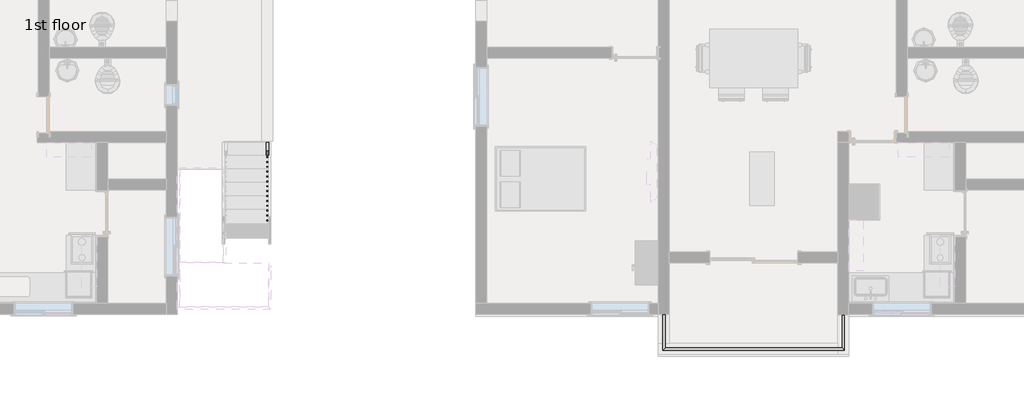
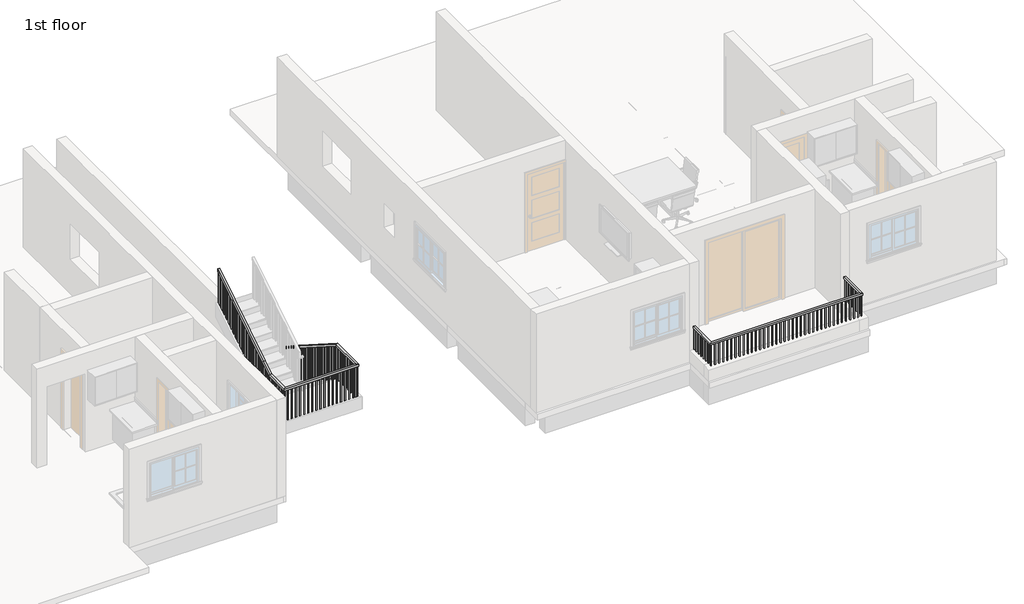
# One storey, part 5 of 8: 2 railings.
"""IFC4 building model written with IfcOpenShell, lengths in millimetres."""

from ifc_helpers import new_model, si_unit, frame, origin, place, context, project, spatial, polyline, outline, extrude, faceted_brep, element, save

model = new_model("IFC4")

# Units and contexts
model_context = context("Model", 3, world=origin())
ifc_project = project(units=[si_unit("LENGTHUNIT", "METRE", prefix="MILLI")], contexts=[model_context])

# Site, building, storey
site = spatial("IfcSite", under=ifc_project)
building = spatial("IfcBuilding", under=site)
storey = spatial("IfcBuildingStorey", under=building, Name="1st floor", Elevation=3810.0)

# Railings
placement = place(None, origin())
element("IfcRailing", 1, ObjectType="Handrail - Rectangular", at=placement, inside=storey, context=model_context, shape_type="SolidModel", body=[
    faceted_brep([(-2736.9993763, -1023.9064015, 4902.2), (-2736.9993763, -1023.9064015, 4841.986276), (-2787.7993763, -1023.9064015, 4841.986276), (-2787.7993763, -1023.9064015, 4902.2), (-2736.9993763, -3538.5064015, 6502.4), (-2736.9993763, -3553.2993964, 6451.6), (-2787.7993763, -3553.2993964, 6451.6), (-2787.7993763, -3538.5064015, 6502.4), (-2736.9993763, -4452.9064015, 6502.4), (-2736.9993763, -4452.9064015, 6451.6), (-2787.7993763, -4402.1064015, 6451.6), (-2787.7993763, -4402.1064015, 6502.4), (-4591.1993763, -4452.9064015, 6502.4), (-4591.1993763, -4452.9064015, 6451.6), (-4540.3993763, -4402.1064015, 6451.6), (-4540.3993763, -4402.1064015, 6502.4), (-4591.1993763, -3817.9064015, 6502.4), (-4591.1993763, -3803.1134066, 6451.6), (-4540.3993763, -3803.1134066, 6451.6), (-4540.3993763, -3817.9064015, 6502.4), (-4591.1993763, -3538.5064015, 6680.2), (-4591.1993763, -3511.2331265, 6637.3419964), (-4540.3993763, -3511.2331265, 6637.3419964), (-4540.3993763, -3538.5064015, 6680.2), (-4591.1993763, -1582.7064015, 7924.8), (-4540.3993763, -1582.7064015, 7924.8), (-4540.3993763, -1582.7064015, 7864.586276), (-4591.1993763, -1582.7064015, 7864.586276)], [[[0, 1, 2, 3]], [[1, 0, 4, 5]], [[2, 1, 5, 6]], [[3, 2, 6, 7]], [[0, 3, 7, 4]], [[5, 4, 8, 9]], [[6, 5, 9, 10]], [[7, 6, 10, 11]], [[4, 7, 11, 8]], [[9, 8, 12, 13]], [[10, 9, 13, 14]], [[11, 10, 14, 15]], [[8, 11, 15, 12]], [[13, 12, 16, 17]], [[14, 13, 17, 18]], [[15, 14, 18, 19]], [[12, 15, 19, 16]], [[17, 16, 20, 21]], [[18, 17, 21, 22]], [[19, 18, 22, 23]], [[16, 19, 23, 20]], [[24, 25, 26, 27]], [[21, 20, 24, 27]], [[22, 21, 27, 26]], [[23, 22, 26, 25]], [[20, 23, 25, 24]]]),
    extrude(outline(polyline([(-1598.5814015, 7854.4840032), (-1598.5814015, 6832.6), (-1617.6314015, 6832.6), (-1617.6314015, 7842.361276), (-1598.5814015, 7854.4840032)])), frame((-4575.3243763, 0.0, 0.0), z_axis=(1.0, 0.0, 0.0), x_axis=(0.0, 1.0, 0.0)), (0.0, 0.0, 1.0), 19.05),
    extrude(outline(polyline([(-1700.1814015, 7789.8294578), (-1700.1814015, 6832.6), (-1719.2314015, 6832.6), (-1719.2314015, 7777.7067305), (-1700.1814015, 7789.8294578)])), frame((-4575.3243763, 0.0, 0.0), z_axis=(1.0, 0.0, 0.0), x_axis=(0.0, 1.0, 0.0)), (0.0, 0.0, 1.0), 19.05),
    extrude(outline(polyline([(-1801.7814015, 7725.1749123), (-1801.7814015, 6832.6), (-1820.8314015, 6832.6), (-1820.8314015, 7713.0521851), (-1801.7814015, 7725.1749123)])), frame((-4575.3243763, 0.0, 0.0), z_axis=(1.0, 0.0, 0.0), x_axis=(0.0, 1.0, 0.0)), (0.0, 0.0, 1.0), 19.05),
    extrude(outline(polyline([(-1903.3814015, 7660.5203669), (-1903.3814015, 6654.8), (-1922.4314015, 6654.8), (-1922.4314015, 7648.3976396), (-1903.3814015, 7660.5203669)])), frame((-4575.3243763, 0.0, 0.0), z_axis=(1.0, 0.0, 0.0), x_axis=(0.0, 1.0, 0.0)), (0.0, 0.0, 1.0), 19.05),
    extrude(outline(polyline([(-2004.9814015, 7595.8658214), (-2004.9814015, 6654.8), (-2024.0314015, 6654.8), (-2024.0314015, 7583.7430941), (-2004.9814015, 7595.8658214)])), frame((-4575.3243763, 0.0, 0.0), z_axis=(1.0, 0.0, 0.0), x_axis=(0.0, 1.0, 0.0)), (0.0, 0.0, 1.0), 19.05),
    extrude(outline(polyline([(-2106.5814015, 7531.211276), (-2106.5814015, 6654.8), (-2125.6314015, 6654.8), (-2125.6314015, 7519.0885487), (-2106.5814015, 7531.211276)])), frame((-4575.3243763, 0.0, 0.0), z_axis=(1.0, 0.0, 0.0), x_axis=(0.0, 1.0, 0.0)), (0.0, 0.0, 1.0), 19.05),
    extrude(outline(polyline([(-2208.1814015, 7466.5567305), (-2208.1814015, 6477.0), (-2227.2314015, 6477.0), (-2227.2314015, 7454.4340032), (-2208.1814015, 7466.5567305)])), frame((-4575.3243763, 0.0, 0.0), z_axis=(1.0, 0.0, 0.0), x_axis=(0.0, 1.0, 0.0)), (0.0, 0.0, 1.0), 19.05),
    extrude(outline(polyline([(-2309.7814015, 7401.9021851), (-2309.7814015, 6477.0), (-2328.8314015, 6477.0), (-2328.8314015, 7389.7794578), (-2309.7814015, 7401.9021851)])), frame((-4575.3243763, 0.0, 0.0), z_axis=(1.0, 0.0, 0.0), x_axis=(0.0, 1.0, 0.0)), (0.0, 0.0, 1.0), 19.05),
    extrude(outline(polyline([(-2411.3814015, 7337.2476396), (-2411.3814015, 6477.0), (-2430.4314015, 6477.0), (-2430.4314015, 7325.1249123), (-2411.3814015, 7337.2476396)])), frame((-4575.3243763, 0.0, 0.0), z_axis=(1.0, 0.0, 0.0), x_axis=(0.0, 1.0, 0.0)), (0.0, 0.0, 1.0), 19.05),
    extrude(outline(polyline([(-2512.9814015, 7272.5930941), (-2512.9814015, 6299.2), (-2532.0314015, 6299.2), (-2532.0314015, 7260.4703669), (-2512.9814015, 7272.5930941)])), frame((-4575.3243763, 0.0, 0.0), z_axis=(1.0, 0.0, 0.0), x_axis=(0.0, 1.0, 0.0)), (0.0, 0.0, 1.0), 19.05),
    extrude(outline(polyline([(-2614.5814015, 7207.9385487), (-2614.5814015, 6299.2), (-2633.6314015, 6299.2), (-2633.6314015, 7195.8158214), (-2614.5814015, 7207.9385487)])), frame((-4575.3243763, 0.0, 0.0), z_axis=(1.0, 0.0, 0.0), x_axis=(0.0, 1.0, 0.0)), (0.0, 0.0, 1.0), 19.05),
    extrude(outline(polyline([(-2716.1814015, 7143.2840032), (-2716.1814015, 6121.4), (-2735.2314015, 6121.4), (-2735.2314015, 7131.161276), (-2716.1814015, 7143.2840032)])), frame((-4575.3243763, 0.0, 0.0), z_axis=(1.0, 0.0, 0.0), x_axis=(0.0, 1.0, 0.0)), (0.0, 0.0, 1.0), 19.05),
    extrude(outline(polyline([(-2817.7814015, 7078.6294578), (-2817.7814015, 6121.4), (-2836.8314015, 6121.4), (-2836.8314015, 7066.5067305), (-2817.7814015, 7078.6294578)])), frame((-4575.3243763, 0.0, 0.0), z_axis=(1.0, 0.0, 0.0), x_axis=(0.0, 1.0, 0.0)), (0.0, 0.0, 1.0), 19.05),
    extrude(outline(polyline([(-2919.3814015, 7013.9749123), (-2919.3814015, 6121.4), (-2938.4314015, 6121.4), (-2938.4314015, 7001.8521851), (-2919.3814015, 7013.9749123)])), frame((-4575.3243763, 0.0, 0.0), z_axis=(1.0, 0.0, 0.0), x_axis=(0.0, 1.0, 0.0)), (0.0, 0.0, 1.0), 19.05),
    extrude(outline(polyline([(-3020.9814015, 6949.3203669), (-3020.9814015, 5943.6), (-3040.0314015, 5943.6), (-3040.0314015, 6937.1976396), (-3020.9814015, 6949.3203669)])), frame((-4575.3243763, 0.0, 0.0), z_axis=(1.0, 0.0, 0.0), x_axis=(0.0, 1.0, 0.0)), (0.0, 0.0, 1.0), 19.05),
    extrude(outline(polyline([(-3122.5814015, 6884.6658214), (-3122.5814015, 5943.6), (-3141.6314015, 5943.6), (-3141.6314015, 6872.5430941), (-3122.5814015, 6884.6658214)])), frame((-4575.3243763, 0.0, 0.0), z_axis=(1.0, 0.0, 0.0), x_axis=(0.0, 1.0, 0.0)), (0.0, 0.0, 1.0), 19.05),
    extrude(outline(polyline([(-3224.1814015, 6820.011276), (-3224.1814015, 5943.6), (-3243.2314015, 5943.6), (-3243.2314015, 6807.8885487), (-3224.1814015, 6820.011276)])), frame((-4575.3243763, 0.0, 0.0), z_axis=(1.0, 0.0, 0.0), x_axis=(0.0, 1.0, 0.0)), (0.0, 0.0, 1.0), 19.05),
    extrude(outline(polyline([(-3325.7814015, 6755.3567305), (-3325.7814015, 5765.8), (-3344.8314015, 5765.8), (-3344.8314015, 6743.2340032), (-3325.7814015, 6755.3567305)])), frame((-4575.3243763, 0.0, 0.0), z_axis=(1.0, 0.0, 0.0), x_axis=(0.0, 1.0, 0.0)), (0.0, 0.0, 1.0), 19.05),
    extrude(outline(polyline([(-3427.3814015, 6690.7021851), (-3427.3814015, 5765.8), (-3446.4314015, 5765.8), (-3446.4314015, 6678.5794578), (-3427.3814015, 6690.7021851)])), frame((-4575.3243763, 0.0, 0.0), z_axis=(1.0, 0.0, 0.0), x_axis=(0.0, 1.0, 0.0)), (0.0, 0.0, 1.0), 19.05),
    extrude(outline(polyline([(-3605.1814015, 6577.5567305), (-3605.1814015, 5588.0), (-3624.2314015, 5588.0), (-3624.2314015, 6565.4340032), (-3605.1814015, 6577.5567305)])), frame((-4575.3243763, 0.0, 0.0), z_axis=(1.0, 0.0, 0.0), x_axis=(0.0, 1.0, 0.0)), (0.0, 0.0, 1.0), 19.05),
    extrude(outline(polyline([(-3706.7814015, 6512.9021851), (-3706.7814015, 5588.0), (-3725.8314015, 5588.0), (-3725.8314015, 6500.7794578), (-3706.7814015, 6512.9021851)])), frame((-4575.3243763, 0.0, 0.0), z_axis=(1.0, 0.0, 0.0), x_axis=(0.0, 1.0, 0.0)), (0.0, 0.0, 1.0), 19.05),
    extrude(outline(polyline([(-4575.3243763, -3827.4314015), (-4575.3243763, -3808.3814015), (-4556.2743763, -3808.3814015), (-4556.2743763, -3827.4314015), (-4575.3243763, -3827.4314015)])), frame((0.0, 0.0, 5588.0), z_axis=(0.0, 0.0, 1.0), x_axis=(1.0, 0.0, 0.0)), (0.0, 0.0, 1.0), 863.6),
    extrude(outline(polyline([(-4575.3243763, -3929.0314015), (-4575.3243763, -3909.9814015), (-4556.2743763, -3909.9814015), (-4556.2743763, -3929.0314015), (-4575.3243763, -3929.0314015)])), frame((0.0, 0.0, 5588.0), z_axis=(0.0, 0.0, 1.0), x_axis=(1.0, 0.0, 0.0)), (0.0, 0.0, 1.0), 863.6),
    extrude(outline(polyline([(-4575.3243763, -4030.6314015), (-4575.3243763, -4011.5814015), (-4556.2743763, -4011.5814015), (-4556.2743763, -4030.6314015), (-4575.3243763, -4030.6314015)])), frame((0.0, 0.0, 5588.0), z_axis=(0.0, 0.0, 1.0), x_axis=(1.0, 0.0, 0.0)), (0.0, 0.0, 1.0), 863.6),
    extrude(outline(polyline([(-4575.3243763, -4132.2314015), (-4575.3243763, -4113.1814015), (-4556.2743763, -4113.1814015), (-4556.2743763, -4132.2314015), (-4575.3243763, -4132.2314015)])), frame((0.0, 0.0, 5588.0), z_axis=(0.0, 0.0, 1.0), x_axis=(1.0, 0.0, 0.0)), (0.0, 0.0, 1.0), 863.6),
    extrude(outline(polyline([(-4575.3243763, -4233.8314015), (-4575.3243763, -4214.7814015), (-4556.2743763, -4214.7814015), (-4556.2743763, -4233.8314015), (-4575.3243763, -4233.8314015)])), frame((0.0, 0.0, 5588.0), z_axis=(0.0, 0.0, 1.0), x_axis=(1.0, 0.0, 0.0)), (0.0, 0.0, 1.0), 863.6),
    extrude(outline(polyline([(-4575.3243763, -4335.4314015), (-4575.3243763, -4316.3814015), (-4556.2743763, -4316.3814015), (-4556.2743763, -4335.4314015), (-4575.3243763, -4335.4314015)])), frame((0.0, 0.0, 5588.0), z_axis=(0.0, 0.0, 1.0), x_axis=(1.0, 0.0, 0.0)), (0.0, 0.0, 1.0), 863.6),
    extrude(outline(polyline([(-4480.0743763, -4437.0314015), (-4499.1243763, -4437.0314015), (-4499.1243763, -4417.9814015), (-4480.0743763, -4417.9814015), (-4480.0743763, -4437.0314015)])), frame((0.0, 0.0, 5588.0), z_axis=(0.0, 0.0, 1.0), x_axis=(1.0, 0.0, 0.0)), (0.0, 0.0, 1.0), 863.6),
    extrude(outline(polyline([(-4378.4743763, -4437.0314015), (-4397.5243763, -4437.0314015), (-4397.5243763, -4417.9814015), (-4378.4743763, -4417.9814015), (-4378.4743763, -4437.0314015)])), frame((0.0, 0.0, 5588.0), z_axis=(0.0, 0.0, 1.0), x_axis=(1.0, 0.0, 0.0)), (0.0, 0.0, 1.0), 863.6),
    extrude(outline(polyline([(-4276.8743763, -4437.0314015), (-4295.9243763, -4437.0314015), (-4295.9243763, -4417.9814015), (-4276.8743763, -4417.9814015), (-4276.8743763, -4437.0314015)])), frame((0.0, 0.0, 5588.0), z_axis=(0.0, 0.0, 1.0), x_axis=(1.0, 0.0, 0.0)), (0.0, 0.0, 1.0), 863.6),
    extrude(outline(polyline([(-4175.2743763, -4437.0314015), (-4194.3243763, -4437.0314015), (-4194.3243763, -4417.9814015), (-4175.2743763, -4417.9814015), (-4175.2743763, -4437.0314015)])), frame((0.0, 0.0, 5588.0), z_axis=(0.0, 0.0, 1.0), x_axis=(1.0, 0.0, 0.0)), (0.0, 0.0, 1.0), 863.6),
    extrude(outline(polyline([(-4073.6743763, -4437.0314015), (-4092.7243763, -4437.0314015), (-4092.7243763, -4417.9814015), (-4073.6743763, -4417.9814015), (-4073.6743763, -4437.0314015)])), frame((0.0, 0.0, 5588.0), z_axis=(0.0, 0.0, 1.0), x_axis=(1.0, 0.0, 0.0)), (0.0, 0.0, 1.0), 863.6),
    extrude(outline(polyline([(-3972.0743763, -4437.0314015), (-3991.1243763, -4437.0314015), (-3991.1243763, -4417.9814015), (-3972.0743763, -4417.9814015), (-3972.0743763, -4437.0314015)])), frame((0.0, 0.0, 5588.0), z_axis=(0.0, 0.0, 1.0), x_axis=(1.0, 0.0, 0.0)), (0.0, 0.0, 1.0), 863.6),
    extrude(outline(polyline([(-3870.4743763, -4437.0314015), (-3889.5243763, -4437.0314015), (-3889.5243763, -4417.9814015), (-3870.4743763, -4417.9814015), (-3870.4743763, -4437.0314015)])), frame((0.0, 0.0, 5588.0), z_axis=(0.0, 0.0, 1.0), x_axis=(1.0, 0.0, 0.0)), (0.0, 0.0, 1.0), 863.6),
    extrude(outline(polyline([(-3768.8743763, -4437.0314015), (-3787.9243763, -4437.0314015), (-3787.9243763, -4417.9814015), (-3768.8743763, -4417.9814015), (-3768.8743763, -4437.0314015)])), frame((0.0, 0.0, 5588.0), z_axis=(0.0, 0.0, 1.0), x_axis=(1.0, 0.0, 0.0)), (0.0, 0.0, 1.0), 863.6),
    extrude(outline(polyline([(-3667.2743763, -4437.0314015), (-3686.3243763, -4437.0314015), (-3686.3243763, -4417.9814015), (-3667.2743763, -4417.9814015), (-3667.2743763, -4437.0314015)])), frame((0.0, 0.0, 5588.0), z_axis=(0.0, 0.0, 1.0), x_axis=(1.0, 0.0, 0.0)), (0.0, 0.0, 1.0), 863.6),
    extrude(outline(polyline([(-3565.6743763, -4437.0314015), (-3584.7243763, -4437.0314015), (-3584.7243763, -4417.9814015), (-3565.6743763, -4417.9814015), (-3565.6743763, -4437.0314015)])), frame((0.0, 0.0, 5588.0), z_axis=(0.0, 0.0, 1.0), x_axis=(1.0, 0.0, 0.0)), (0.0, 0.0, 1.0), 863.6),
    extrude(outline(polyline([(-3464.0743763, -4437.0314015), (-3483.1243763, -4437.0314015), (-3483.1243763, -4417.9814015), (-3464.0743763, -4417.9814015), (-3464.0743763, -4437.0314015)])), frame((0.0, 0.0, 5588.0), z_axis=(0.0, 0.0, 1.0), x_axis=(1.0, 0.0, 0.0)), (0.0, 0.0, 1.0), 863.6),
    extrude(outline(polyline([(-3362.4743763, -4437.0314015), (-3381.5243763, -4437.0314015), (-3381.5243763, -4417.9814015), (-3362.4743763, -4417.9814015), (-3362.4743763, -4437.0314015)])), frame((0.0, 0.0, 5588.0), z_axis=(0.0, 0.0, 1.0), x_axis=(1.0, 0.0, 0.0)), (0.0, 0.0, 1.0), 863.6),
    extrude(outline(polyline([(-3260.8743763, -4437.0314015), (-3279.9243763, -4437.0314015), (-3279.9243763, -4417.9814015), (-3260.8743763, -4417.9814015), (-3260.8743763, -4437.0314015)])), frame((0.0, 0.0, 5588.0), z_axis=(0.0, 0.0, 1.0), x_axis=(1.0, 0.0, 0.0)), (0.0, 0.0, 1.0), 863.6),
    extrude(outline(polyline([(-3159.2743763, -4437.0314015), (-3178.3243763, -4437.0314015), (-3178.3243763, -4417.9814015), (-3159.2743763, -4417.9814015), (-3159.2743763, -4437.0314015)])), frame((0.0, 0.0, 5588.0), z_axis=(0.0, 0.0, 1.0), x_axis=(1.0, 0.0, 0.0)), (0.0, 0.0, 1.0), 863.6),
    extrude(outline(polyline([(-3057.6743763, -4437.0314015), (-3076.7243763, -4437.0314015), (-3076.7243763, -4417.9814015), (-3057.6743763, -4417.9814015), (-3057.6743763, -4437.0314015)])), frame((0.0, 0.0, 5588.0), z_axis=(0.0, 0.0, 1.0), x_axis=(1.0, 0.0, 0.0)), (0.0, 0.0, 1.0), 863.6),
    extrude(outline(polyline([(-2956.0743763, -4437.0314015), (-2975.1243763, -4437.0314015), (-2975.1243763, -4417.9814015), (-2956.0743763, -4417.9814015), (-2956.0743763, -4437.0314015)])), frame((0.0, 0.0, 5588.0), z_axis=(0.0, 0.0, 1.0), x_axis=(1.0, 0.0, 0.0)), (0.0, 0.0, 1.0), 863.6),
    extrude(outline(polyline([(-2854.4743763, -4437.0314015), (-2873.5243763, -4437.0314015), (-2873.5243763, -4417.9814015), (-2854.4743763, -4417.9814015), (-2854.4743763, -4437.0314015)])), frame((0.0, 0.0, 5588.0), z_axis=(0.0, 0.0, 1.0), x_axis=(1.0, 0.0, 0.0)), (0.0, 0.0, 1.0), 863.6),
    extrude(outline(polyline([(-2752.8743763, -4341.7814015), (-2752.8743763, -4360.8314015), (-2771.9243763, -4360.8314015), (-2771.9243763, -4341.7814015), (-2752.8743763, -4341.7814015)])), frame((0.0, 0.0, 5588.0), z_axis=(0.0, 0.0, 1.0), x_axis=(1.0, 0.0, 0.0)), (0.0, 0.0, 1.0), 863.6),
    extrude(outline(polyline([(-2752.8743763, -4240.1814015), (-2752.8743763, -4259.2314015), (-2771.9243763, -4259.2314015), (-2771.9243763, -4240.1814015), (-2752.8743763, -4240.1814015)])), frame((0.0, 0.0, 5588.0), z_axis=(0.0, 0.0, 1.0), x_axis=(1.0, 0.0, 0.0)), (0.0, 0.0, 1.0), 863.6),
    extrude(outline(polyline([(-2752.8743763, -4138.5814015), (-2752.8743763, -4157.6314015), (-2771.9243763, -4157.6314015), (-2771.9243763, -4138.5814015), (-2752.8743763, -4138.5814015)])), frame((0.0, 0.0, 5588.0), z_axis=(0.0, 0.0, 1.0), x_axis=(1.0, 0.0, 0.0)), (0.0, 0.0, 1.0), 863.6),
    extrude(outline(polyline([(-2752.8743763, -4036.9814015), (-2752.8743763, -4056.0314015), (-2771.9243763, -4056.0314015), (-2771.9243763, -4036.9814015), (-2752.8743763, -4036.9814015)])), frame((0.0, 0.0, 5588.0), z_axis=(0.0, 0.0, 1.0), x_axis=(1.0, 0.0, 0.0)), (0.0, 0.0, 1.0), 863.6),
    extrude(outline(polyline([(-2752.8743763, -3935.3814015), (-2752.8743763, -3954.4314015), (-2771.9243763, -3954.4314015), (-2771.9243763, -3935.3814015), (-2752.8743763, -3935.3814015)])), frame((0.0, 0.0, 5588.0), z_axis=(0.0, 0.0, 1.0), x_axis=(1.0, 0.0, 0.0)), (0.0, 0.0, 1.0), 863.6),
    extrude(outline(polyline([(-2752.8743763, -3833.7814015), (-2752.8743763, -3852.8314015), (-2771.9243763, -3852.8314015), (-2771.9243763, -3833.7814015), (-2752.8743763, -3833.7814015)])), frame((0.0, 0.0, 5588.0), z_axis=(0.0, 0.0, 1.0), x_axis=(1.0, 0.0, 0.0)), (0.0, 0.0, 1.0), 863.6),
    extrude(outline(polyline([(-2752.8743763, -3732.1814015), (-2752.8743763, -3751.2314015), (-2771.9243763, -3751.2314015), (-2771.9243763, -3732.1814015), (-2752.8743763, -3732.1814015)])), frame((0.0, 0.0, 5588.0), z_axis=(0.0, 0.0, 1.0), x_axis=(1.0, 0.0, 0.0)), (0.0, 0.0, 1.0), 863.6),
    extrude(outline(polyline([(-2752.8743763, -3630.5814015), (-2752.8743763, -3649.6314015), (-2771.9243763, -3649.6314015), (-2771.9243763, -3630.5814015), (-2752.8743763, -3630.5814015)])), frame((0.0, 0.0, 5588.0), z_axis=(0.0, 0.0, 1.0), x_axis=(1.0, 0.0, 0.0)), (0.0, 0.0, 1.0), 863.6),
    extrude(outline(polyline([(-3452.7814015, 6387.6340032), (-3452.7814015, 5410.2), (-3471.8314015, 5410.2), (-3471.8314015, 6399.7567305), (-3452.7814015, 6387.6340032)])), frame((-2771.9243763, 0.0, 0.0), z_axis=(1.0, 0.0, 0.0), x_axis=(0.0, 1.0, 0.0)), (0.0, 0.0, 1.0), 19.05),
    extrude(outline(polyline([(-3351.1814015, 6322.9794578), (-3351.1814015, 5410.2), (-3370.2314015, 5410.2), (-3370.2314015, 6335.1021851), (-3351.1814015, 6322.9794578)])), frame((-2771.9243763, 0.0, 0.0), z_axis=(1.0, 0.0, 0.0), x_axis=(0.0, 1.0, 0.0)), (0.0, 0.0, 1.0), 19.05),
    extrude(outline(polyline([(-3249.5814015, 6258.3249123), (-3249.5814015, 5410.2), (-3268.6314015, 5410.2), (-3268.6314015, 6270.4476396), (-3249.5814015, 6258.3249123)])), frame((-2771.9243763, 0.0, 0.0), z_axis=(1.0, 0.0, 0.0), x_axis=(0.0, 1.0, 0.0)), (0.0, 0.0, 1.0), 19.05),
    extrude(outline(polyline([(-3147.9814015, 6193.6703669), (-3147.9814015, 5232.4), (-3167.0314015, 5232.4), (-3167.0314015, 6205.7930941), (-3147.9814015, 6193.6703669)])), frame((-2771.9243763, 0.0, 0.0), z_axis=(1.0, 0.0, 0.0), x_axis=(0.0, 1.0, 0.0)), (0.0, 0.0, 1.0), 19.05),
    extrude(outline(polyline([(-3046.3814015, 6129.0158214), (-3046.3814015, 5232.4), (-3065.4314015, 5232.4), (-3065.4314015, 6141.1385487), (-3046.3814015, 6129.0158214)])), frame((-2771.9243763, 0.0, 0.0), z_axis=(1.0, 0.0, 0.0), x_axis=(0.0, 1.0, 0.0)), (0.0, 0.0, 1.0), 19.05),
    extrude(outline(polyline([(-2944.7814015, 6064.361276), (-2944.7814015, 5054.6), (-2963.8314015, 5054.6), (-2963.8314015, 6076.4840032), (-2944.7814015, 6064.361276)])), frame((-2771.9243763, 0.0, 0.0), z_axis=(1.0, 0.0, 0.0), x_axis=(0.0, 1.0, 0.0)), (0.0, 0.0, 1.0), 19.05),
    extrude(outline(polyline([(-2843.1814015, 5999.7067305), (-2843.1814015, 5054.6), (-2862.2314015, 5054.6), (-2862.2314015, 6011.8294578), (-2843.1814015, 5999.7067305)])), frame((-2771.9243763, 0.0, 0.0), z_axis=(1.0, 0.0, 0.0), x_axis=(0.0, 1.0, 0.0)), (0.0, 0.0, 1.0), 19.05),
    extrude(outline(polyline([(-2741.5814015, 5935.0521851), (-2741.5814015, 5054.6), (-2760.6314015, 5054.6), (-2760.6314015, 5947.1749123), (-2741.5814015, 5935.0521851)])), frame((-2771.9243763, 0.0, 0.0), z_axis=(1.0, 0.0, 0.0), x_axis=(0.0, 1.0, 0.0)), (0.0, 0.0, 1.0), 19.05),
    extrude(outline(polyline([(-2639.9814015, 5870.3976396), (-2639.9814015, 4876.8), (-2659.0314015, 4876.8), (-2659.0314015, 5882.5203669), (-2639.9814015, 5870.3976396)])), frame((-2771.9243763, 0.0, 0.0), z_axis=(1.0, 0.0, 0.0), x_axis=(0.0, 1.0, 0.0)), (0.0, 0.0, 1.0), 19.05),
    extrude(outline(polyline([(-2538.3814015, 5805.7430941), (-2538.3814015, 4876.8), (-2557.4314015, 4876.8), (-2557.4314015, 5817.8658214), (-2538.3814015, 5805.7430941)])), frame((-2771.9243763, 0.0, 0.0), z_axis=(1.0, 0.0, 0.0), x_axis=(0.0, 1.0, 0.0)), (0.0, 0.0, 1.0), 19.05),
    extrude(outline(polyline([(-2436.7814015, 5741.0885487), (-2436.7814015, 4876.8), (-2455.8314015, 4876.8), (-2455.8314015, 5753.211276), (-2436.7814015, 5741.0885487)])), frame((-2771.9243763, 0.0, 0.0), z_axis=(1.0, 0.0, 0.0), x_axis=(0.0, 1.0, 0.0)), (0.0, 0.0, 1.0), 19.05),
    extrude(outline(polyline([(-2335.1814015, 5676.4340032), (-2335.1814015, 4699.0), (-2354.2314015, 4699.0), (-2354.2314015, 5688.5567305), (-2335.1814015, 5676.4340032)])), frame((-2771.9243763, 0.0, 0.0), z_axis=(1.0, 0.0, 0.0), x_axis=(0.0, 1.0, 0.0)), (0.0, 0.0, 1.0), 19.05),
    extrude(outline(polyline([(-2233.5814015, 5611.7794578), (-2233.5814015, 4699.0), (-2252.6314015, 4699.0), (-2252.6314015, 5623.9021851), (-2233.5814015, 5611.7794578)])), frame((-2771.9243763, 0.0, 0.0), z_axis=(1.0, 0.0, 0.0), x_axis=(0.0, 1.0, 0.0)), (0.0, 0.0, 1.0), 19.05),
    extrude(outline(polyline([(-2131.9814015, 5547.1249123), (-2131.9814015, 4699.0), (-2151.0314015, 4699.0), (-2151.0314015, 5559.2476396), (-2131.9814015, 5547.1249123)])), frame((-2771.9243763, 0.0, 0.0), z_axis=(1.0, 0.0, 0.0), x_axis=(0.0, 1.0, 0.0)), (0.0, 0.0, 1.0), 19.05),
    extrude(outline(polyline([(-2030.3814015, 5482.4703669), (-2030.3814015, 4521.2), (-2049.4314015, 4521.2), (-2049.4314015, 5494.5930941), (-2030.3814015, 5482.4703669)])), frame((-2771.9243763, 0.0, 0.0), z_axis=(1.0, 0.0, 0.0), x_axis=(0.0, 1.0, 0.0)), (0.0, 0.0, 1.0), 19.05),
    extrude(outline(polyline([(-1928.7814015, 5417.8158214), (-1928.7814015, 4521.2), (-1947.8314015, 4521.2), (-1947.8314015, 5429.9385487), (-1928.7814015, 5417.8158214)])), frame((-2771.9243763, 0.0, 0.0), z_axis=(1.0, 0.0, 0.0), x_axis=(0.0, 1.0, 0.0)), (0.0, 0.0, 1.0), 19.05),
    extrude(outline(polyline([(-1827.1814015, 5353.161276), (-1827.1814015, 4343.4), (-1846.2314015, 4343.4), (-1846.2314015, 5365.2840032), (-1827.1814015, 5353.161276)])), frame((-2771.9243763, 0.0, 0.0), z_axis=(1.0, 0.0, 0.0), x_axis=(0.0, 1.0, 0.0)), (0.0, 0.0, 1.0), 19.05),
    extrude(outline(polyline([(-1725.5814015, 5288.5067305), (-1725.5814015, 4343.4), (-1744.6314015, 4343.4), (-1744.6314015, 5300.6294578), (-1725.5814015, 5288.5067305)])), frame((-2771.9243763, 0.0, 0.0), z_axis=(1.0, 0.0, 0.0), x_axis=(0.0, 1.0, 0.0)), (0.0, 0.0, 1.0), 19.05),
    extrude(outline(polyline([(-1623.9814015, 5223.8521851), (-1623.9814015, 4343.4), (-1643.0314015, 4343.4), (-1643.0314015, 5235.9749123), (-1623.9814015, 5223.8521851)])), frame((-2771.9243763, 0.0, 0.0), z_axis=(1.0, 0.0, 0.0), x_axis=(0.0, 1.0, 0.0)), (0.0, 0.0, 1.0), 19.05),
    extrude(outline(polyline([(-1522.3814015, 5159.1976396), (-1522.3814015, 4165.6), (-1541.4314015, 4165.6), (-1541.4314015, 5171.3203669), (-1522.3814015, 5159.1976396)])), frame((-2771.9243763, 0.0, 0.0), z_axis=(1.0, 0.0, 0.0), x_axis=(0.0, 1.0, 0.0)), (0.0, 0.0, 1.0), 19.05),
    extrude(outline(polyline([(-1420.7814015, 5094.5430941), (-1420.7814015, 4165.6), (-1439.8314015, 4165.6), (-1439.8314015, 5106.6658214), (-1420.7814015, 5094.5430941)])), frame((-2771.9243763, 0.0, 0.0), z_axis=(1.0, 0.0, 0.0), x_axis=(0.0, 1.0, 0.0)), (0.0, 0.0, 1.0), 19.05),
    extrude(outline(polyline([(-1319.1814015, 5029.8885487), (-1319.1814015, 4165.6), (-1338.2314015, 4165.6), (-1338.2314015, 5042.011276), (-1319.1814015, 5029.8885487)])), frame((-2771.9243763, 0.0, 0.0), z_axis=(1.0, 0.0, 0.0), x_axis=(0.0, 1.0, 0.0)), (0.0, 0.0, 1.0), 19.05),
    extrude(outline(polyline([(-1217.5814015, 4965.2340032), (-1217.5814015, 3987.8), (-1236.6314015, 3987.8), (-1236.6314015, 4977.3567305), (-1217.5814015, 4965.2340032)])), frame((-2771.9243763, 0.0, 0.0), z_axis=(1.0, 0.0, 0.0), x_axis=(0.0, 1.0, 0.0)), (0.0, 0.0, 1.0), 19.05),
    extrude(outline(polyline([(-1115.9814015, 4900.5794578), (-1115.9814015, 3987.8), (-1135.0314015, 3987.8), (-1135.0314015, 4912.7021851), (-1115.9814015, 4900.5794578)])), frame((-2771.9243763, 0.0, 0.0), z_axis=(1.0, 0.0, 0.0), x_axis=(0.0, 1.0, 0.0)), (0.0, 0.0, 1.0), 19.05),
    extrude(outline(polyline([(-3528.9814015, 6626.0476396), (-3528.9814015, 5588.0), (-3548.0314015, 5588.0), (-3548.0314015, 6613.9249123), (-3528.9814015, 6626.0476396)])), frame((-4575.3243763, 0.0, 0.0), z_axis=(1.0, 0.0, 0.0), x_axis=(0.0, 1.0, 0.0)), (0.0, 0.0, 1.0), 19.05),
    extrude(outline(polyline([(-4556.2743763, -4437.0314015), (-4575.3243763, -4437.0314015), (-4575.3243763, -4417.9814015), (-4556.2743763, -4417.9814015), (-4556.2743763, -4437.0314015)])), frame((0.0, 0.0, 5588.0), z_axis=(0.0, 0.0, 1.0), x_axis=(1.0, 0.0, 0.0)), (0.0, 0.0, 1.0), 863.6),
    extrude(outline(polyline([(-2752.8743763, -4417.9814015), (-2752.8743763, -4437.0314015), (-2771.9243763, -4437.0314015), (-2771.9243763, -4417.9814015), (-2752.8743763, -4417.9814015)])), frame((0.0, 0.0, 5588.0), z_axis=(0.0, 0.0, 1.0), x_axis=(1.0, 0.0, 0.0)), (0.0, 0.0, 1.0), 863.6),
    extrude(outline(polyline([(-3528.9814015, 6436.1249123), (-3528.9814015, 5588.0), (-3548.0314015, 5588.0), (-3548.0314015, 6448.2476396), (-3528.9814015, 6436.1249123)])), frame((-2771.9243763, 0.0, 0.0), z_axis=(1.0, 0.0, 0.0), x_axis=(0.0, 1.0, 0.0)), (0.0, 0.0, 1.0), 19.05),
    extrude(outline(polyline([(-1582.7064015, 7864.586276), (-1582.7064015, 6832.6), (-1601.7564015, 6832.6), (-1601.7564015, 7852.4635487), (-1582.7064015, 7864.586276)])), frame((-4575.3243763, 0.0, 0.0), z_axis=(1.0, 0.0, 0.0), x_axis=(0.0, 1.0, 0.0)), (0.0, 0.0, 1.0), 19.05),
    extrude(outline(polyline([(-1023.9064015, 4841.986276), (-1023.9064015, 3987.8), (-1042.9564015, 3987.8), (-1042.9564015, 4854.1090032), (-1023.9064015, 4841.986276)])), frame((-2771.9243763, 0.0, 0.0), z_axis=(1.0, 0.0, 0.0), x_axis=(0.0, 1.0, 0.0)), (0.0, 0.0, 1.0), 19.05),
])
element("IfcRailing", 2, ObjectType="Handrail - Rectangular", at=placement, inside=storey, context=model_context, shape_type="SolidModel", body=[
    faceted_brep([(5523.6761273, -4611.6564015, 4724.4), (5523.6761273, -4611.6564015, 4673.6), (5472.8761273, -4611.6564015, 4673.6), (5472.8761273, -4611.6564015, 4724.4), (5523.6761273, -5303.8064015, 4724.4), (5523.6761273, -5303.8064015, 4673.6), (5472.8761273, -5354.6064015, 4673.6), (5472.8761273, -5354.6064015, 4724.4), (9206.6761273, -5303.8064015, 4724.4), (9206.6761273, -5303.8064015, 4673.6), (9257.4761273, -5354.6064015, 4673.6), (9257.4761273, -5354.6064015, 4724.4), (9206.6761273, -4618.0064015, 4724.4), (9257.4761273, -4618.0064015, 4724.4), (9257.4761273, -4618.0064015, 4673.6), (9206.6761273, -4618.0064015, 4673.6)], [[[0, 1, 2, 3]], [[1, 0, 4, 5]], [[2, 1, 5, 6]], [[3, 2, 6, 7]], [[0, 3, 7, 4]], [[5, 4, 8, 9]], [[6, 5, 9, 10]], [[7, 6, 10, 11]], [[4, 7, 11, 8]], [[12, 13, 14, 15]], [[9, 8, 12, 15]], [[10, 9, 15, 14]], [[11, 10, 14, 13]], [[8, 11, 13, 12]]]),
    extrude(outline(polyline([(9241.6011273, -4729.1314015), (9222.5511273, -4729.1314015), (9222.5511273, -4710.0814015), (9241.6011273, -4710.0814015), (9241.6011273, -4729.1314015)])), frame((0.0, 0.0, 3810.0), z_axis=(0.0, 0.0, 1.0), x_axis=(1.0, 0.0, 0.0)), (0.0, 0.0, 1.0), 863.6),
    extrude(outline(polyline([(9241.6011273, -4830.7314015), (9222.5511273, -4830.7314015), (9222.5511273, -4811.6814015), (9241.6011273, -4811.6814015), (9241.6011273, -4830.7314015)])), frame((0.0, 0.0, 3810.0), z_axis=(0.0, 0.0, 1.0), x_axis=(1.0, 0.0, 0.0)), (0.0, 0.0, 1.0), 863.6),
    extrude(outline(polyline([(9241.6011273, -4932.3314015), (9222.5511273, -4932.3314015), (9222.5511273, -4913.2814015), (9241.6011273, -4913.2814015), (9241.6011273, -4932.3314015)])), frame((0.0, 0.0, 3810.0), z_axis=(0.0, 0.0, 1.0), x_axis=(1.0, 0.0, 0.0)), (0.0, 0.0, 1.0), 863.6),
    extrude(outline(polyline([(9241.6011273, -5033.9314015), (9222.5511273, -5033.9314015), (9222.5511273, -5014.8814015), (9241.6011273, -5014.8814015), (9241.6011273, -5033.9314015)])), frame((0.0, 0.0, 3810.0), z_axis=(0.0, 0.0, 1.0), x_axis=(1.0, 0.0, 0.0)), (0.0, 0.0, 1.0), 863.6),
    extrude(outline(polyline([(9241.6011273, -5135.5314015), (9222.5511273, -5135.5314015), (9222.5511273, -5116.4814015), (9241.6011273, -5116.4814015), (9241.6011273, -5135.5314015)])), frame((0.0, 0.0, 3810.0), z_axis=(0.0, 0.0, 1.0), x_axis=(1.0, 0.0, 0.0)), (0.0, 0.0, 1.0), 863.6),
    extrude(outline(polyline([(9241.6011273, -5237.1314015), (9222.5511273, -5237.1314015), (9222.5511273, -5218.0814015), (9241.6011273, -5218.0814015), (9241.6011273, -5237.1314015)])), frame((0.0, 0.0, 3810.0), z_axis=(0.0, 0.0, 1.0), x_axis=(1.0, 0.0, 0.0)), (0.0, 0.0, 1.0), 863.6),
    extrude(outline(polyline([(9146.3511273, -5338.7314015), (9146.3511273, -5319.6814015), (9165.4011273, -5319.6814015), (9165.4011273, -5338.7314015), (9146.3511273, -5338.7314015)])), frame((0.0, 0.0, 3810.0), z_axis=(0.0, 0.0, 1.0), x_axis=(1.0, 0.0, 0.0)), (0.0, 0.0, 1.0), 863.6),
    extrude(outline(polyline([(9044.7511273, -5338.7314015), (9044.7511273, -5319.6814015), (9063.8011273, -5319.6814015), (9063.8011273, -5338.7314015), (9044.7511273, -5338.7314015)])), frame((0.0, 0.0, 3810.0), z_axis=(0.0, 0.0, 1.0), x_axis=(1.0, 0.0, 0.0)), (0.0, 0.0, 1.0), 863.6),
    extrude(outline(polyline([(8943.1511273, -5338.7314015), (8943.1511273, -5319.6814015), (8962.2011273, -5319.6814015), (8962.2011273, -5338.7314015), (8943.1511273, -5338.7314015)])), frame((0.0, 0.0, 3810.0), z_axis=(0.0, 0.0, 1.0), x_axis=(1.0, 0.0, 0.0)), (0.0, 0.0, 1.0), 863.6),
    extrude(outline(polyline([(8841.5511273, -5338.7314015), (8841.5511273, -5319.6814015), (8860.6011273, -5319.6814015), (8860.6011273, -5338.7314015), (8841.5511273, -5338.7314015)])), frame((0.0, 0.0, 3810.0), z_axis=(0.0, 0.0, 1.0), x_axis=(1.0, 0.0, 0.0)), (0.0, 0.0, 1.0), 863.6),
    extrude(outline(polyline([(8739.9511273, -5338.7314015), (8739.9511273, -5319.6814015), (8759.0011273, -5319.6814015), (8759.0011273, -5338.7314015), (8739.9511273, -5338.7314015)])), frame((0.0, 0.0, 3810.0), z_axis=(0.0, 0.0, 1.0), x_axis=(1.0, 0.0, 0.0)), (0.0, 0.0, 1.0), 863.6),
    extrude(outline(polyline([(8638.3511273, -5338.7314015), (8638.3511273, -5319.6814015), (8657.4011273, -5319.6814015), (8657.4011273, -5338.7314015), (8638.3511273, -5338.7314015)])), frame((0.0, 0.0, 3810.0), z_axis=(0.0, 0.0, 1.0), x_axis=(1.0, 0.0, 0.0)), (0.0, 0.0, 1.0), 863.6),
    extrude(outline(polyline([(8536.7511273, -5338.7314015), (8536.7511273, -5319.6814015), (8555.8011273, -5319.6814015), (8555.8011273, -5338.7314015), (8536.7511273, -5338.7314015)])), frame((0.0, 0.0, 3810.0), z_axis=(0.0, 0.0, 1.0), x_axis=(1.0, 0.0, 0.0)), (0.0, 0.0, 1.0), 863.6),
    extrude(outline(polyline([(8435.1511273, -5338.7314015), (8435.1511273, -5319.6814015), (8454.2011273, -5319.6814015), (8454.2011273, -5338.7314015), (8435.1511273, -5338.7314015)])), frame((0.0, 0.0, 3810.0), z_axis=(0.0, 0.0, 1.0), x_axis=(1.0, 0.0, 0.0)), (0.0, 0.0, 1.0), 863.6),
    extrude(outline(polyline([(8333.5511273, -5338.7314015), (8333.5511273, -5319.6814015), (8352.6011273, -5319.6814015), (8352.6011273, -5338.7314015), (8333.5511273, -5338.7314015)])), frame((0.0, 0.0, 3810.0), z_axis=(0.0, 0.0, 1.0), x_axis=(1.0, 0.0, 0.0)), (0.0, 0.0, 1.0), 863.6),
    extrude(outline(polyline([(8231.9511273, -5338.7314015), (8231.9511273, -5319.6814015), (8251.0011273, -5319.6814015), (8251.0011273, -5338.7314015), (8231.9511273, -5338.7314015)])), frame((0.0, 0.0, 3810.0), z_axis=(0.0, 0.0, 1.0), x_axis=(1.0, 0.0, 0.0)), (0.0, 0.0, 1.0), 863.6),
    extrude(outline(polyline([(8130.3511273, -5338.7314015), (8130.3511273, -5319.6814015), (8149.4011273, -5319.6814015), (8149.4011273, -5338.7314015), (8130.3511273, -5338.7314015)])), frame((0.0, 0.0, 3810.0), z_axis=(0.0, 0.0, 1.0), x_axis=(1.0, 0.0, 0.0)), (0.0, 0.0, 1.0), 863.6),
    extrude(outline(polyline([(8028.7511273, -5338.7314015), (8028.7511273, -5319.6814015), (8047.8011273, -5319.6814015), (8047.8011273, -5338.7314015), (8028.7511273, -5338.7314015)])), frame((0.0, 0.0, 3810.0), z_axis=(0.0, 0.0, 1.0), x_axis=(1.0, 0.0, 0.0)), (0.0, 0.0, 1.0), 863.6),
    extrude(outline(polyline([(7927.1511273, -5338.7314015), (7927.1511273, -5319.6814015), (7946.2011273, -5319.6814015), (7946.2011273, -5338.7314015), (7927.1511273, -5338.7314015)])), frame((0.0, 0.0, 3810.0), z_axis=(0.0, 0.0, 1.0), x_axis=(1.0, 0.0, 0.0)), (0.0, 0.0, 1.0), 863.6),
    extrude(outline(polyline([(7825.5511273, -5338.7314015), (7825.5511273, -5319.6814015), (7844.6011273, -5319.6814015), (7844.6011273, -5338.7314015), (7825.5511273, -5338.7314015)])), frame((0.0, 0.0, 3810.0), z_axis=(0.0, 0.0, 1.0), x_axis=(1.0, 0.0, 0.0)), (0.0, 0.0, 1.0), 863.6),
    extrude(outline(polyline([(7723.9511273, -5338.7314015), (7723.9511273, -5319.6814015), (7743.0011273, -5319.6814015), (7743.0011273, -5338.7314015), (7723.9511273, -5338.7314015)])), frame((0.0, 0.0, 3810.0), z_axis=(0.0, 0.0, 1.0), x_axis=(1.0, 0.0, 0.0)), (0.0, 0.0, 1.0), 863.6),
    extrude(outline(polyline([(7622.3511273, -5338.7314015), (7622.3511273, -5319.6814015), (7641.4011273, -5319.6814015), (7641.4011273, -5338.7314015), (7622.3511273, -5338.7314015)])), frame((0.0, 0.0, 3810.0), z_axis=(0.0, 0.0, 1.0), x_axis=(1.0, 0.0, 0.0)), (0.0, 0.0, 1.0), 863.6),
    extrude(outline(polyline([(7520.7511273, -5338.7314015), (7520.7511273, -5319.6814015), (7539.8011273, -5319.6814015), (7539.8011273, -5338.7314015), (7520.7511273, -5338.7314015)])), frame((0.0, 0.0, 3810.0), z_axis=(0.0, 0.0, 1.0), x_axis=(1.0, 0.0, 0.0)), (0.0, 0.0, 1.0), 863.6),
    extrude(outline(polyline([(7419.1511273, -5338.7314015), (7419.1511273, -5319.6814015), (7438.2011273, -5319.6814015), (7438.2011273, -5338.7314015), (7419.1511273, -5338.7314015)])), frame((0.0, 0.0, 3810.0), z_axis=(0.0, 0.0, 1.0), x_axis=(1.0, 0.0, 0.0)), (0.0, 0.0, 1.0), 863.6),
    extrude(outline(polyline([(7317.5511273, -5338.7314015), (7317.5511273, -5319.6814015), (7336.6011273, -5319.6814015), (7336.6011273, -5338.7314015), (7317.5511273, -5338.7314015)])), frame((0.0, 0.0, 3810.0), z_axis=(0.0, 0.0, 1.0), x_axis=(1.0, 0.0, 0.0)), (0.0, 0.0, 1.0), 863.6),
    extrude(outline(polyline([(7215.9511273, -5338.7314015), (7215.9511273, -5319.6814015), (7235.0011273, -5319.6814015), (7235.0011273, -5338.7314015), (7215.9511273, -5338.7314015)])), frame((0.0, 0.0, 3810.0), z_axis=(0.0, 0.0, 1.0), x_axis=(1.0, 0.0, 0.0)), (0.0, 0.0, 1.0), 863.6),
    extrude(outline(polyline([(7114.3511273, -5338.7314015), (7114.3511273, -5319.6814015), (7133.4011273, -5319.6814015), (7133.4011273, -5338.7314015), (7114.3511273, -5338.7314015)])), frame((0.0, 0.0, 3810.0), z_axis=(0.0, 0.0, 1.0), x_axis=(1.0, 0.0, 0.0)), (0.0, 0.0, 1.0), 863.6),
    extrude(outline(polyline([(7012.7511273, -5338.7314015), (7012.7511273, -5319.6814015), (7031.8011273, -5319.6814015), (7031.8011273, -5338.7314015), (7012.7511273, -5338.7314015)])), frame((0.0, 0.0, 3810.0), z_axis=(0.0, 0.0, 1.0), x_axis=(1.0, 0.0, 0.0)), (0.0, 0.0, 1.0), 863.6),
    extrude(outline(polyline([(6911.1511273, -5338.7314015), (6911.1511273, -5319.6814015), (6930.2011273, -5319.6814015), (6930.2011273, -5338.7314015), (6911.1511273, -5338.7314015)])), frame((0.0, 0.0, 3810.0), z_axis=(0.0, 0.0, 1.0), x_axis=(1.0, 0.0, 0.0)), (0.0, 0.0, 1.0), 863.6),
    extrude(outline(polyline([(6809.5511273, -5338.7314015), (6809.5511273, -5319.6814015), (6828.6011273, -5319.6814015), (6828.6011273, -5338.7314015), (6809.5511273, -5338.7314015)])), frame((0.0, 0.0, 3810.0), z_axis=(0.0, 0.0, 1.0), x_axis=(1.0, 0.0, 0.0)), (0.0, 0.0, 1.0), 863.6),
    extrude(outline(polyline([(6707.9511273, -5338.7314015), (6707.9511273, -5319.6814015), (6727.0011273, -5319.6814015), (6727.0011273, -5338.7314015), (6707.9511273, -5338.7314015)])), frame((0.0, 0.0, 3810.0), z_axis=(0.0, 0.0, 1.0), x_axis=(1.0, 0.0, 0.0)), (0.0, 0.0, 1.0), 863.6),
    extrude(outline(polyline([(6606.3511273, -5338.7314015), (6606.3511273, -5319.6814015), (6625.4011273, -5319.6814015), (6625.4011273, -5338.7314015), (6606.3511273, -5338.7314015)])), frame((0.0, 0.0, 3810.0), z_axis=(0.0, 0.0, 1.0), x_axis=(1.0, 0.0, 0.0)), (0.0, 0.0, 1.0), 863.6),
    extrude(outline(polyline([(6504.7511273, -5338.7314015), (6504.7511273, -5319.6814015), (6523.8011273, -5319.6814015), (6523.8011273, -5338.7314015), (6504.7511273, -5338.7314015)])), frame((0.0, 0.0, 3810.0), z_axis=(0.0, 0.0, 1.0), x_axis=(1.0, 0.0, 0.0)), (0.0, 0.0, 1.0), 863.6),
    extrude(outline(polyline([(6403.1511273, -5338.7314015), (6403.1511273, -5319.6814015), (6422.2011273, -5319.6814015), (6422.2011273, -5338.7314015), (6403.1511273, -5338.7314015)])), frame((0.0, 0.0, 3810.0), z_axis=(0.0, 0.0, 1.0), x_axis=(1.0, 0.0, 0.0)), (0.0, 0.0, 1.0), 863.6),
    extrude(outline(polyline([(6301.5511273, -5338.7314015), (6301.5511273, -5319.6814015), (6320.6011273, -5319.6814015), (6320.6011273, -5338.7314015), (6301.5511273, -5338.7314015)])), frame((0.0, 0.0, 3810.0), z_axis=(0.0, 0.0, 1.0), x_axis=(1.0, 0.0, 0.0)), (0.0, 0.0, 1.0), 863.6),
    extrude(outline(polyline([(6199.9511273, -5338.7314015), (6199.9511273, -5319.6814015), (6219.0011273, -5319.6814015), (6219.0011273, -5338.7314015), (6199.9511273, -5338.7314015)])), frame((0.0, 0.0, 3810.0), z_axis=(0.0, 0.0, 1.0), x_axis=(1.0, 0.0, 0.0)), (0.0, 0.0, 1.0), 863.6),
    extrude(outline(polyline([(6098.3511273, -5338.7314015), (6098.3511273, -5319.6814015), (6117.4011273, -5319.6814015), (6117.4011273, -5338.7314015), (6098.3511273, -5338.7314015)])), frame((0.0, 0.0, 3810.0), z_axis=(0.0, 0.0, 1.0), x_axis=(1.0, 0.0, 0.0)), (0.0, 0.0, 1.0), 863.6),
    extrude(outline(polyline([(5996.7511273, -5338.7314015), (5996.7511273, -5319.6814015), (6015.8011273, -5319.6814015), (6015.8011273, -5338.7314015), (5996.7511273, -5338.7314015)])), frame((0.0, 0.0, 3810.0), z_axis=(0.0, 0.0, 1.0), x_axis=(1.0, 0.0, 0.0)), (0.0, 0.0, 1.0), 863.6),
    extrude(outline(polyline([(5895.1511273, -5338.7314015), (5895.1511273, -5319.6814015), (5914.2011273, -5319.6814015), (5914.2011273, -5338.7314015), (5895.1511273, -5338.7314015)])), frame((0.0, 0.0, 3810.0), z_axis=(0.0, 0.0, 1.0), x_axis=(1.0, 0.0, 0.0)), (0.0, 0.0, 1.0), 863.6),
    extrude(outline(polyline([(5793.5511273, -5338.7314015), (5793.5511273, -5319.6814015), (5812.6011273, -5319.6814015), (5812.6011273, -5338.7314015), (5793.5511273, -5338.7314015)])), frame((0.0, 0.0, 3810.0), z_axis=(0.0, 0.0, 1.0), x_axis=(1.0, 0.0, 0.0)), (0.0, 0.0, 1.0), 863.6),
    extrude(outline(polyline([(5691.9511273, -5338.7314015), (5691.9511273, -5319.6814015), (5711.0011273, -5319.6814015), (5711.0011273, -5338.7314015), (5691.9511273, -5338.7314015)])), frame((0.0, 0.0, 3810.0), z_axis=(0.0, 0.0, 1.0), x_axis=(1.0, 0.0, 0.0)), (0.0, 0.0, 1.0), 863.6),
    extrude(outline(polyline([(5590.3511273, -5338.7314015), (5590.3511273, -5319.6814015), (5609.4011273, -5319.6814015), (5609.4011273, -5338.7314015), (5590.3511273, -5338.7314015)])), frame((0.0, 0.0, 3810.0), z_axis=(0.0, 0.0, 1.0), x_axis=(1.0, 0.0, 0.0)), (0.0, 0.0, 1.0), 863.6),
    extrude(outline(polyline([(5488.7511273, -5313.3314015), (5507.8011273, -5313.3314015), (5507.8011273, -5332.3814015), (5488.7511273, -5332.3814015), (5488.7511273, -5313.3314015)])), frame((0.0, 0.0, 3810.0), z_axis=(0.0, 0.0, 1.0), x_axis=(1.0, 0.0, 0.0)), (0.0, 0.0, 1.0), 863.6),
    extrude(outline(polyline([(5488.7511273, -5211.7314015), (5507.8011273, -5211.7314015), (5507.8011273, -5230.7814015), (5488.7511273, -5230.7814015), (5488.7511273, -5211.7314015)])), frame((0.0, 0.0, 3810.0), z_axis=(0.0, 0.0, 1.0), x_axis=(1.0, 0.0, 0.0)), (0.0, 0.0, 1.0), 863.6),
    extrude(outline(polyline([(5488.7511273, -5110.1314015), (5507.8011273, -5110.1314015), (5507.8011273, -5129.1814015), (5488.7511273, -5129.1814015), (5488.7511273, -5110.1314015)])), frame((0.0, 0.0, 3810.0), z_axis=(0.0, 0.0, 1.0), x_axis=(1.0, 0.0, 0.0)), (0.0, 0.0, 1.0), 863.6),
    extrude(outline(polyline([(5488.7511273, -5008.5314015), (5507.8011273, -5008.5314015), (5507.8011273, -5027.5814015), (5488.7511273, -5027.5814015), (5488.7511273, -5008.5314015)])), frame((0.0, 0.0, 3810.0), z_axis=(0.0, 0.0, 1.0), x_axis=(1.0, 0.0, 0.0)), (0.0, 0.0, 1.0), 863.6),
    extrude(outline(polyline([(5488.7511273, -4906.9314015), (5507.8011273, -4906.9314015), (5507.8011273, -4925.9814015), (5488.7511273, -4925.9814015), (5488.7511273, -4906.9314015)])), frame((0.0, 0.0, 3810.0), z_axis=(0.0, 0.0, 1.0), x_axis=(1.0, 0.0, 0.0)), (0.0, 0.0, 1.0), 863.6),
    extrude(outline(polyline([(5488.7511273, -4805.3314015), (5507.8011273, -4805.3314015), (5507.8011273, -4824.3814015), (5488.7511273, -4824.3814015), (5488.7511273, -4805.3314015)])), frame((0.0, 0.0, 3810.0), z_axis=(0.0, 0.0, 1.0), x_axis=(1.0, 0.0, 0.0)), (0.0, 0.0, 1.0), 863.6),
    extrude(outline(polyline([(5488.7511273, -4703.7314015), (5507.8011273, -4703.7314015), (5507.8011273, -4722.7814015), (5488.7511273, -4722.7814015), (5488.7511273, -4703.7314015)])), frame((0.0, 0.0, 3810.0), z_axis=(0.0, 0.0, 1.0), x_axis=(1.0, 0.0, 0.0)), (0.0, 0.0, 1.0), 863.6),
    extrude(outline(polyline([(9222.5511273, -5338.7314015), (9222.5511273, -5319.6814015), (9241.6011273, -5319.6814015), (9241.6011273, -5338.7314015), (9222.5511273, -5338.7314015)])), frame((0.0, 0.0, 3810.0), z_axis=(0.0, 0.0, 1.0), x_axis=(1.0, 0.0, 0.0)), (0.0, 0.0, 1.0), 863.6),
    extrude(outline(polyline([(5488.7511273, -5319.6814015), (5507.8011273, -5319.6814015), (5507.8011273, -5338.7314015), (5488.7511273, -5338.7314015), (5488.7511273, -5319.6814015)])), frame((0.0, 0.0, 3810.0), z_axis=(0.0, 0.0, 1.0), x_axis=(1.0, 0.0, 0.0)), (0.0, 0.0, 1.0), 863.6),
    extrude(outline(polyline([(9241.6011273, -4637.0564015), (9222.5511273, -4637.0564015), (9222.5511273, -4618.0064015), (9241.6011273, -4618.0064015), (9241.6011273, -4637.0564015)])), frame((0.0, 0.0, 3810.0), z_axis=(0.0, 0.0, 1.0), x_axis=(1.0, 0.0, 0.0)), (0.0, 0.0, 1.0), 863.6),
    extrude(outline(polyline([(5488.7511273, -4611.6564015), (5507.8011273, -4611.6564015), (5507.8011273, -4630.7064015), (5488.7511273, -4630.7064015), (5488.7511273, -4611.6564015)])), frame((0.0, 0.0, 3810.0), z_axis=(0.0, 0.0, 1.0), x_axis=(1.0, 0.0, 0.0)), (0.0, 0.0, 1.0), 863.6),
])

save(model, "model.ifc")

# Revit data of these elements
# Type "Handrail - Rectangular"
#   Assembly Code = "C2010400"
#   built-in parameter 1008612 = 0.0416667 (stored number, unit not read)
#   built-in parameter 1008611 = 0.0416667 (stored number, unit not read)
#   built-in parameter 1008609 = 0.333333 (stored number, unit not read)
#   built-in parameter 1008604 = 0.166667 (stored number, unit not read)
#   built-in parameter 1008603 = 0.166667 (stored number, unit not read)
#   Railing Height = 3' - 0"
#   built-in parameter 1008630 = 2
#   built-in parameter 1008610 = 2
#   built-in parameter 1008618 = Baluster - Square : 3/4"
# Elements 1, 2 (IfcRailing, "Handrail - Rectangular")
#   Phase Created = New Construction
